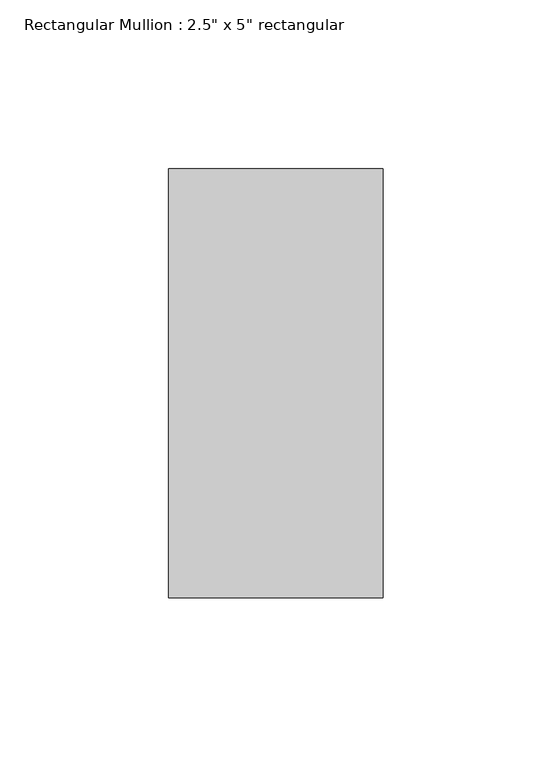
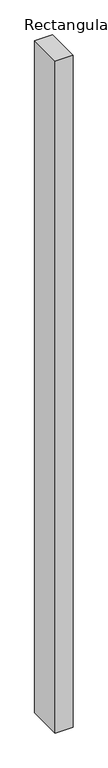
"""IFC4 building model written with IfcOpenShell, lengths in millimetres: member geometry."""

from ifc_helpers import new_model, si_unit, frame, origin, place, context, project, spatial, polyline, outline, extrude, source, transform, mapped, element, save


def member_4863f604(model_context):
    return source(origin(), model_context, "Body", "SweptSolid", [
        extrude(outline(polyline([(0.0, 63.5), (0.0, -63.5), (-63.5, -63.5), (-63.5, 63.5), (0.0, 63.5)])), frame((0.0, 0.0, -2529.4963211), z_axis=(0.0, 0.0, 1.0), x_axis=(1.0, 0.0, 0.0)), (0.0, 0.0, 1.0), 2529.4963211),
    ])


if __name__ == "__main__":
    model = new_model("IFC4")
    model_context = context("Model", 3, world=origin())
    ifc_project = project(units=[si_unit("LENGTHUNIT", "METRE", prefix="MILLI")], contexts=[model_context])
    site = spatial("IfcSite", under=ifc_project)
    building = spatial("IfcBuilding", under=site)
    placement = place(None, origin())
    member_shape = member_4863f604(model_context)
    element("IfcMember", 1, ObjectType="Rectangular Mullion : 2.5\" x 5\" rectangular", at=placement, inside=building, context=model_context, shape_type="MappedRepresentation", body=[
        mapped(member_shape, transform((0.0, 0.0, 0.0), x_axis=(1.0, 0.0, 0.0), y_axis=(0.0, 1.0, 0.0), z_axis=(0.0, 0.0, 1.0))),
    ])
    save(model, "model.ifc")

# Revit data of these elements
# Type "Rectangular Mullion : 2.5\" x 5\" rectangular"
#   built-in parameter 1007304 = 0.416667 (stored number, unit not read)
#   built-in parameter 1007301 = 0.104167 (stored number, unit not read)
#   built-in parameter 1007300 = 0.104167 (stored number, unit not read)
# Element 1 (IfcMember, "Rectangular Mullion : 2.5\" x 5\" rectangular")
#   Materials on its faces: "Aluminum"
# Materials
#   "Aluminum": class "Metal", colour RGB 247 247 247, transparency 0, Description = "Aluminum 6061", Cost = 0
